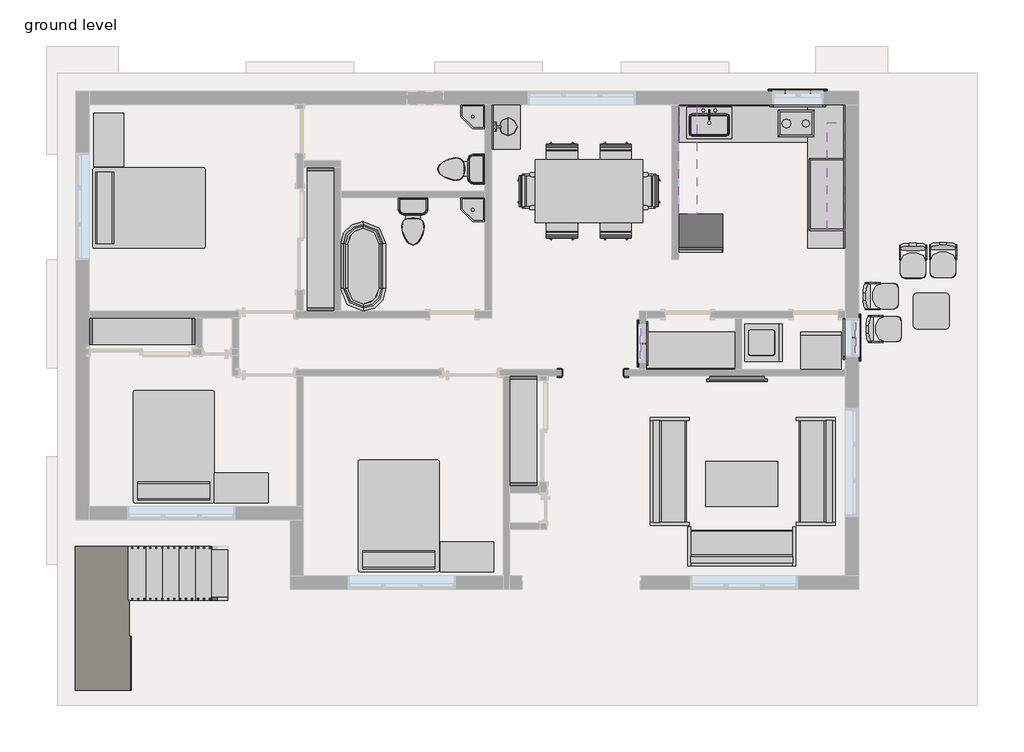
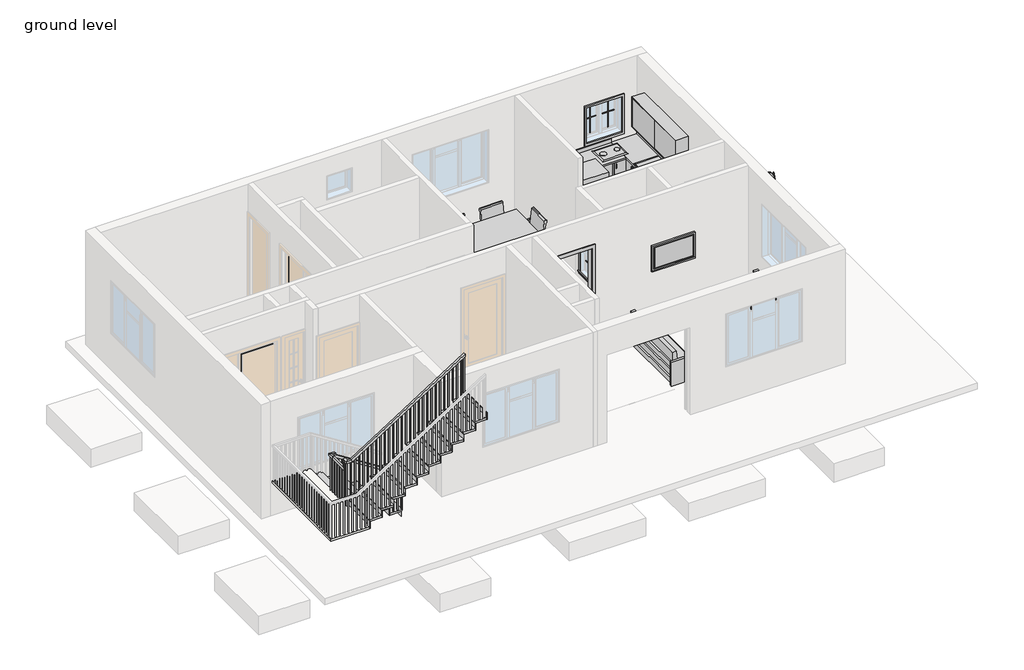
# One storey, part 4 of 4: 34 furniture elements, 17 proxies, 7 flow terminals, 2 stair flights, 1 railing, 1 slab.
"""IFC4 building model written with IfcOpenShell, lengths in millimetres."""

from ifc_helpers import new_model, si_unit, frame, origin, place, context, project, spatial, polyline, outline, extrude, faceted_brep, transform, mapped, element, save
from components import proxy_3c1fa1d0, proxy_97c73763, muntin_pattern_2x2_muntin_pattern_2x2_b3fe6957, muntin_pattern_2x2_muntin_pattern_2x2_3e0ecaf2, muntin_pattern_2x2_muntin_pattern_2x2_c35c595f, muntin_pattern_2x2_muntin_pattern_2x2_183aef24, proxy_bc9927fa, proxy_e6cf46b9, trim_window_exterior_flat_with_sill_41619996, trim_window_exterior_flat_with_sill_e38017c9, trim_window_exterior_flat_with_sill_5e960bf5, trim_window_interior_flat_picture_frame_51c85655, trim_window_interior_flat_picture_frame_d728ed12, trim_window_interior_flat_picture_frame_80babb00, proxy_1934c8a4, flow_terminal_15267b2a, flow_terminal_5b58e753, flow_terminal_4d548711, toilet_domestic_3d_toilet_domestic_3d_ba6479b0, toilet_domestic_3d_toilet_domestic_3d_30431060, flow_terminal_ce36f001, furniture_48488436, furniture_f87f75a4, furniture_97fe820d, furniture_52ef1662, furniture_6b884072, chair_task_chair_task_b7f3823b, chair_task_arms_chair_task_arms_fa5a08ef, furniture_deb1c5d1, furniture_9388d8e7, furniture_74614b7d, furniture_eb3a3c23, furniture_53a00f75, furniture_df918c0e, furniture_57be741f, furniture_57f9710a, furniture_acc2807d, furniture_65ba067b, furniture_5d68651d, furniture_b6aab1a0, furniture_1cc80a06, non_monolithic_landing_1ab817cb, stair_flight_17170d3d, stair_flight_b41fd25d

model = new_model("IFC4")

# Units and contexts
model_context = context("Model", 3, world=origin())
ifc_project = project(units=[si_unit("LENGTHUNIT", "METRE", prefix="MILLI")], contexts=[model_context])

# Site, building, storey
site = spatial("IfcSite", under=ifc_project)
building = spatial("IfcBuilding", under=site)
storey = spatial("IfcBuildingStorey", under=building, Name="ground level", Elevation=609.6)

# Proxies
placement = place(None, origin())
proxy_shape = proxy_3c1fa1d0(model_context)
element("IfcBuildingElementProxy", 1, Name="Cook Top-2 Unit : 12\" x 18\"", ObjectType="Cook Top-2 Unit : 12\" x 18\"", at=placement, inside=storey, context=model_context, shape_type="MappedRepresentation", body=[
    mapped(proxy_shape, transform((3099.7984427, 6060.3661978, 609.6), x_axis=(0.0, 1.0, 0.0), y_axis=(-1.0, 0.0, 0.0), z_axis=(0.0, 0.0, 1.0))),
])
proxy_2_shape = proxy_97c73763(model_context)
element("IfcBuildingElementProxy", 2, Name="Dryer : 27\" x 25\" x 35\"", ObjectType="Dryer : 27\" x 25\" x 35\"", at=placement, inside=storey, context=model_context, shape_type="MappedRepresentation", body=[
    mapped(proxy_2_shape, transform((3116.0361908, 1961.105194, 609.6), x_axis=(1.0, 0.0, 0.0), y_axis=(0.0, 1.0, 0.0), z_axis=(0.0, 0.0, 1.0))),
])
muntin_pattern_2x2_muntin_pattern_2x2_shape = muntin_pattern_2x2_muntin_pattern_2x2_b3fe6957(model_context)
element("IfcBuildingElementProxy", 3, Name="Muntin Pattern_2x2 : Muntin Pattern_2x2", ObjectType="Muntin Pattern_2x2 : Muntin Pattern_2x2", at=placement, inside=storey, context=model_context, shape_type="MappedRepresentation", body=[
    mapped(muntin_pattern_2x2_muntin_pattern_2x2_shape, transform((2887.0111471, 6673.1411978, 1771.65), x_axis=(1.0, 0.0, 0.0), y_axis=(0.0, 1.0, 0.0), z_axis=(0.0, 0.0, 1.0))),
])
muntin_pattern_2x2_muntin_pattern_2x2_2_shape = muntin_pattern_2x2_muntin_pattern_2x2_3e0ecaf2(model_context)
element("IfcBuildingElementProxy", 4, Name="Muntin Pattern_2x2 : Muntin Pattern_2x2", ObjectType="Muntin Pattern_2x2 : Muntin Pattern_2x2", at=placement, inside=storey, context=model_context, shape_type="MappedRepresentation", body=[
    mapped(muntin_pattern_2x2_muntin_pattern_2x2_2_shape, transform((3315.6361471, 6673.1411978, 1771.65), x_axis=(-1.0, 0.0, 0.0), y_axis=(0.0, -1.0, 0.0), z_axis=(0.0, 0.0, 1.0))),
])
muntin_pattern_2x2_muntin_pattern_2x2_3_shape = muntin_pattern_2x2_muntin_pattern_2x2_c35c595f(model_context)
element("IfcBuildingElementProxy", 5, Name="Muntin Pattern_2x2 : Muntin Pattern_2x2", ObjectType="Muntin Pattern_2x2 : Muntin Pattern_2x2", at=placement, inside=storey, context=model_context, shape_type="MappedRepresentation", body=[
    mapped(muntin_pattern_2x2_muntin_pattern_2x2_3_shape, transform((4095.0986471, 2498.0161978, 2079.625), x_axis=(0.0, -1.0, 0.0), y_axis=(1.0, 0.0, 0.0), z_axis=(0.0, 0.0, 1.0))),
])
element("IfcBuildingElementProxy", 6, Name="Muntin Pattern_2x2 : Muntin Pattern_2x2", ObjectType="Muntin Pattern_2x2 : Muntin Pattern_2x2", at=placement, inside=storey, context=model_context, shape_type="MappedRepresentation", body=[
    mapped(muntin_pattern_2x2_muntin_pattern_2x2_3_shape, transform((4050.6486471, 2498.0161978, 1600.2), x_axis=(0.0, -1.0, 0.0), y_axis=(1.0, 0.0, 0.0), z_axis=(0.0, 0.0, 1.0))),
])
muntin_pattern_2x2_muntin_pattern_2x2_4_shape = muntin_pattern_2x2_muntin_pattern_2x2_183aef24(model_context)
element("IfcBuildingElementProxy", 7, Name="Muntin Pattern_2x2 : Muntin Pattern_2x2", ObjectType="Muntin Pattern_2x2 : Muntin Pattern_2x2", at=placement, inside=storey, context=model_context, shape_type="MappedRepresentation", body=[
    mapped(muntin_pattern_2x2_muntin_pattern_2x2_4_shape, transform((443.8486471, 2396.4161978, 2079.625), x_axis=(0.0, -1.0, 0.0), y_axis=(1.0, 0.0, 0.0), z_axis=(0.0, 0.0, 1.0))),
])
element("IfcBuildingElementProxy", 8, Name="Muntin Pattern_2x2 : Muntin Pattern_2x2", ObjectType="Muntin Pattern_2x2 : Muntin Pattern_2x2", at=placement, inside=storey, context=model_context, shape_type="MappedRepresentation", body=[
    mapped(muntin_pattern_2x2_muntin_pattern_2x2_4_shape, transform((488.2986471, 2396.4161978, 1600.2), x_axis=(0.0, -1.0, 0.0), y_axis=(1.0, 0.0, 0.0), z_axis=(0.0, 0.0, 1.0))),
])
proxy_3_shape = proxy_bc9927fa(model_context)
element("IfcBuildingElementProxy", 9, Name="Passage Opening-Cased : 36\" x 84\"", ObjectType="Passage Opening-Cased : 36\" x 84\"", at=placement, inside=storey, context=model_context, shape_type="MappedRepresentation", body=[
    mapped(proxy_3_shape, transform((-386.6650096, 1901.1161978, 609.6), x_axis=(-1.0, 0.0, 0.0), y_axis=(0.0, -1.0, 0.0), z_axis=(0.0, 0.0, 1.0))),
])
proxy_4_shape = proxy_e6cf46b9(model_context)
element("IfcBuildingElementProxy", 10, Name="Refrigerator-Built-in : 30\" x 24\" RH", ObjectType="Refrigerator-Built-in : 30\" x 24\" RH", at=placement, inside=storey, context=model_context, shape_type="MappedRepresentation", body=[
    mapped(proxy_4_shape, transform((1450.3236471, 4309.7422263, 609.6), x_axis=(1.0, 0.0, 0.0), y_axis=(0.0, 1.0, 0.0), z_axis=(0.0, 0.0, 1.0))),
])
trim_window_exterior_flat_with_sill_shape = trim_window_exterior_flat_with_sill_41619996(model_context)
element("IfcBuildingElementProxy", 11, Name="Trim-Window-Exterior-Flat : with Sill", ObjectType="Trim-Window-Exterior-Flat : with Sill", at=placement, inside=storey, context=model_context, shape_type="MappedRepresentation", body=[
    mapped(trim_window_exterior_flat_with_sill_shape, transform((3101.3236471, 6682.6661978, 2616.2), x_axis=(-1.0, 0.0, 0.0), y_axis=(0.0, 0.0, 1.0), z_axis=(0.0, 1.0, 0.0))),
])
trim_window_exterior_flat_with_sill_2_shape = trim_window_exterior_flat_with_sill_e38017c9(model_context)
element("IfcBuildingElementProxy", 12, Name="Trim-Window-Exterior-Flat : with Sill", ObjectType="Trim-Window-Exterior-Flat : with Sill", at=placement, inside=storey, context=model_context, shape_type="MappedRepresentation", body=[
    mapped(trim_window_exterior_flat_with_sill_2_shape, transform((4130.0236471, 2498.0161978, 2590.8), x_axis=(0.0, 1.0, 0.0), y_axis=(0.0, 0.0, 1.0), z_axis=(1.0, 0.0, 0.0))),
])
trim_window_exterior_flat_with_sill_3_shape = trim_window_exterior_flat_with_sill_5e960bf5(model_context)
element("IfcBuildingElementProxy", 13, Name="Trim-Window-Exterior-Flat : with Sill", ObjectType="Trim-Window-Exterior-Flat : with Sill", at=placement, inside=storey, context=model_context, shape_type="MappedRepresentation", body=[
    mapped(trim_window_exterior_flat_with_sill_3_shape, transform((408.9236471, 2396.4161978, 2590.8), x_axis=(0.0, 1.0, 0.0), y_axis=(0.0, 0.0, -1.0), z_axis=(-1.0, 0.0, 0.0))),
])
trim_window_interior_flat_picture_frame_shape = trim_window_interior_flat_picture_frame_51c85655(model_context)
element("IfcBuildingElementProxy", 14, Name="Trim-Window-Interior-Flat : Picture Frame", ObjectType="Trim-Window-Interior-Flat : Picture Frame", at=placement, inside=storey, context=model_context, shape_type="MappedRepresentation", body=[
    mapped(trim_window_interior_flat_picture_frame_shape, transform((3101.3236471, 6454.0661978, 2616.2), x_axis=(1.0, 0.0, 0.0), y_axis=(0.0, 0.0, 1.0), z_axis=(0.0, -1.0, 0.0))),
])
trim_window_interior_flat_picture_frame_2_shape = trim_window_interior_flat_picture_frame_d728ed12(model_context)
element("IfcBuildingElementProxy", 15, Name="Trim-Window-Interior-Flat : Picture Frame", ObjectType="Trim-Window-Interior-Flat : Picture Frame", at=placement, inside=storey, context=model_context, shape_type="MappedRepresentation", body=[
    mapped(trim_window_interior_flat_picture_frame_2_shape, transform((3901.4236471, 2498.0161978, 2590.8), x_axis=(0.0, -1.0, 0.0), y_axis=(0.0, 0.0, 1.0), z_axis=(-1.0, 0.0, 0.0))),
])
trim_window_interior_flat_picture_frame_3_shape = trim_window_interior_flat_picture_frame_80babb00(model_context)
element("IfcBuildingElementProxy", 16, Name="Trim-Window-Interior-Flat : Picture Frame", ObjectType="Trim-Window-Interior-Flat : Picture Frame", at=placement, inside=storey, context=model_context, shape_type="MappedRepresentation", body=[
    mapped(trim_window_interior_flat_picture_frame_3_shape, transform((523.2236471, 2396.4161978, 2590.8), x_axis=(0.0, -1.0, 0.0), y_axis=(0.0, 0.0, -1.0), z_axis=(1.0, 0.0, 0.0))),
])
proxy_5_shape = proxy_1934c8a4(model_context)
element("IfcBuildingElementProxy", 17, Name="Washer : 25\" x 25\" x 35\"", ObjectType="Washer : 25\" x 25\" x 35\"", at=placement, inside=storey, context=model_context, shape_type="MappedRepresentation", body=[
    mapped(proxy_5_shape, transform((2237.9740823, 2809.1661978, 609.6), x_axis=(0.0, -1.0, 0.0), y_axis=(1.0, 0.0, 0.0), z_axis=(0.0, 0.0, 1.0))),
])

# Flow terminals
flow_terminal_shape = flow_terminal_15267b2a(model_context)
element("IfcFlowTerminal", 18, ObjectType="Lavatory - Vanity : 30\"x18\" - Private", at=placement, inside=storey, context=model_context, shape_type="MappedRepresentation", body=[
    mapped(flow_terminal_shape, transform((-2099.3263529, 6079.4161978, 609.6), x_axis=(1.0, 0.0, 0.0), y_axis=(0.0, 1.0, 0.0), z_axis=(0.0, 0.0, 1.0))),
])
flow_terminal_2_shape = flow_terminal_5b58e753(model_context)
element("IfcFlowTerminal", 19, ObjectType="Sink - Mop : 28\"x28\"", at=placement, inside=storey, context=model_context, shape_type="MappedRepresentation", body=[
    mapped(flow_terminal_2_shape, transform((-2213.6263529, 4872.9161978, 609.6), x_axis=(0.0, -1.0, 0.0), y_axis=(1.0, 0.0, 0.0), z_axis=(0.0, 0.0, 1.0))),
])
element("IfcFlowTerminal", 20, ObjectType="Sink - Mop : 28\"x28\"", at=placement, inside=storey, context=model_context, shape_type="MappedRepresentation", body=[
    mapped(flow_terminal_2_shape, transform((-2213.6263529, 6454.0661978, 609.6), x_axis=(0.0, -1.0, 0.0), y_axis=(1.0, 0.0, 0.0), z_axis=(0.0, 0.0, 1.0))),
])
flow_terminal_3_shape = flow_terminal_4d548711(model_context)
element("IfcFlowTerminal", 21, ObjectType="Sink Kitchen-Single : 30\" x 21\"", at=placement, inside=storey, context=model_context, shape_type="MappedRepresentation", body=[
    mapped(flow_terminal_3_shape, transform((1580.6844065, 6146.9207967, 609.6), x_axis=(1.0, 0.0, 0.0), y_axis=(0.0, 1.0, 0.0), z_axis=(0.0, 0.0, 1.0))),
])
toilet_domestic_3d_toilet_domestic_3d_shape = toilet_domestic_3d_toilet_domestic_3d_ba6479b0(model_context)
toilet_domestic_3d_toilet_domestic_3d_2_shape = toilet_domestic_3d_toilet_domestic_3d_30431060(model_context)
element("IfcFlowTerminal", 22, ObjectType="Toilet-Domestic-3D : Toilet-Domestic-3D", at=placement, inside=storey, context=model_context, shape_type="MappedRepresentation", body=[
    mapped(toilet_domestic_3d_toilet_domestic_3d_shape, transform((-3433.7493286, 4378.2201704, 609.6), x_axis=(1.0, 0.0, 0.0), y_axis=(0.0, 1.0, 0.0), z_axis=(0.0, 0.0, 1.0))),
    mapped(toilet_domestic_3d_toilet_domestic_3d_2_shape, transform((-3433.7493286, 4378.2201704, 609.6), x_axis=(1.0, 0.0, 0.0), y_axis=(0.0, 1.0, 0.0), z_axis=(0.0, 0.0, 1.0))),
])
element("IfcFlowTerminal", 23, ObjectType="Toilet-Domestic-3D : Toilet-Domestic-3D", at=placement, inside=storey, context=model_context, shape_type="MappedRepresentation", body=[
    mapped(toilet_domestic_3d_toilet_domestic_3d_shape, transform((-2708.3223803, 5361.8661978, 609.6), x_axis=(0.0, -1.0, 0.0), y_axis=(1.0, 0.0, 0.0), z_axis=(0.0, 0.0, 1.0))),
    mapped(toilet_domestic_3d_toilet_domestic_3d_2_shape, transform((-2708.3223803, 5361.8661978, 609.6), x_axis=(0.0, -1.0, 0.0), y_axis=(1.0, 0.0, 0.0), z_axis=(0.0, 0.0, 1.0))),
])
flow_terminal_4_shape = flow_terminal_ce36f001(model_context)
element("IfcFlowTerminal", 24, ObjectType="Tub-Free Standing-3D : 30\" x 60\"", at=placement, inside=storey, context=model_context, shape_type="MappedRepresentation", body=[
    mapped(flow_terminal_4_shape, transform((-4277.3763529, 3710.8661978, 609.6), x_axis=(-1.0, 0.0, 0.0), y_axis=(0.0, -1.0, 0.0), z_axis=(0.0, 0.0, 1.0))),
])

# Furniture
furniture_shape = furniture_48488436(model_context)
element("IfcFurniture", 25, ObjectType="48\"", at=placement, inside=storey, context=model_context, shape_type="MappedRepresentation", body=[
    mapped(furniture_shape, transform((3901.4236471, 5020.9111578, 609.6), x_axis=(0.0, -1.0, 0.0), y_axis=(1.0, 0.0, 0.0), z_axis=(0.0, 0.0, 1.0))),
])
furniture_2_shape = furniture_f87f75a4(model_context)
element("IfcFurniture", 26, ObjectType="Base Cabinet-Combo01 : 30\"", at=placement, inside=storey, context=model_context, shape_type="MappedRepresentation", body=[
    mapped(furniture_2_shape, transform((2587.2859422, 6454.0661978, 609.6), x_axis=(1.0, 0.0, 0.0), y_axis=(0.0, 1.0, 0.0), z_axis=(0.0, 0.0, 1.0))),
])
furniture_3_shape = furniture_97fe820d(model_context)
element("IfcFurniture", 27, ObjectType="Base Cabinet-Corner Unit-Square : 36\"", at=placement, inside=storey, context=model_context, shape_type="MappedRepresentation", body=[
    mapped(furniture_3_shape, transform((3374.6859422, 6454.0661978, 609.6), x_axis=(1.0, 0.0, 0.0), y_axis=(0.0, 1.0, 0.0), z_axis=(0.0, 0.0, 1.0))),
])
furniture_4_shape = furniture_52ef1662(model_context)
element("IfcFurniture", 28, ObjectType="Bed-Standard : Double 54\" x 75\"", at=placement, inside=storey, context=model_context, shape_type="MappedRepresentation", body=[
    mapped(furniture_4_shape, transform((-7961.5214349, 4429.9776732, 609.6), x_axis=(0.0, 1.0, 0.0), y_axis=(-1.0, 0.0, 0.0), z_axis=(0.0, 0.0, 1.0))),
])
element("IfcFurniture", 29, ObjectType="Bed-Standard : Double 54\" x 75\"", at=placement, inside=storey, context=model_context, shape_type="MappedRepresentation", body=[
    mapped(furniture_4_shape, transform((-7225.3378283, 598.2211158, 609.6), x_axis=(-1.0, 0.0, 0.0), y_axis=(0.0, -1.0, 0.0), z_axis=(0.0, 0.0, 1.0))),
])
element("IfcFurniture", 30, ObjectType="Bed-Standard : Double 54\" x 75\"", at=placement, inside=storey, context=model_context, shape_type="MappedRepresentation", body=[
    mapped(furniture_4_shape, transform((-3402.6378283, -576.5288842, 609.6), x_axis=(-1.0, 0.0, 0.0), y_axis=(0.0, -1.0, 0.0), z_axis=(0.0, 0.0, 1.0))),
])
furniture_5_shape = furniture_6b884072(model_context)
element("IfcFurniture", 31, ObjectType="Cabinet File-Lateral 2 Drawer : 36\" x 20\" x 24\"", at=placement, inside=storey, context=model_context, shape_type="MappedRepresentation", body=[
    mapped(furniture_5_shape, transform((-9536.044729, 6037.1887117, 609.6), x_axis=(0.0, 1.0, 0.0), y_axis=(-1.0, 0.0, 0.0), z_axis=(0.0, 0.0, 1.0))),
])
element("IfcFurniture", 32, ObjectType="Cabinet File-Lateral 2 Drawer : 36\" x 20\" x 24\"", at=placement, inside=storey, context=model_context, shape_type="MappedRepresentation", body=[
    mapped(furniture_5_shape, transform((-6527.4988668, -989.0021783, 609.6), x_axis=(-1.0, 0.0, 0.0), y_axis=(0.0, -1.0, 0.0), z_axis=(0.0, 0.0, 1.0))),
])
element("IfcFurniture", 33, ObjectType="Cabinet File-Lateral 2 Drawer : 36\" x 20\" x 24\"", at=placement, inside=storey, context=model_context, shape_type="MappedRepresentation", body=[
    mapped(furniture_5_shape, transform((-2698.4488668, -2163.7521783, 609.6), x_axis=(-1.0, 0.0, 0.0), y_axis=(0.0, -1.0, 0.0), z_axis=(0.0, 0.0, 1.0))),
])
chair_task_chair_task_shape = chair_task_chair_task_b7f3823b(model_context)
element("IfcFurniture", 34, ObjectType="Chair-Task : Chair-Task", at=placement, inside=storey, context=model_context, shape_type="MappedRepresentation", body=[
    mapped(chair_task_chair_task_shape, transform((149.8644668, 5539.5620994, 609.6), x_axis=(-1.0, 0.0, 0.0), y_axis=(0.0, -1.0, 0.0), z_axis=(0.0, 0.0, 1.0))),
])
element("IfcFurniture", 35, ObjectType="Chair-Task : Chair-Task", at=placement, inside=storey, context=model_context, shape_type="MappedRepresentation", body=[
    mapped(chair_task_chair_task_shape, transform((-132.1171726, 4434.8702962, 609.6), x_axis=(1.0, 0.0, 0.0), y_axis=(0.0, 1.0, 0.0), z_axis=(0.0, 0.0, 1.0))),
])
element("IfcFurniture", 36, ObjectType="Chair-Task : Chair-Task", at=placement, inside=storey, context=model_context, shape_type="MappedRepresentation", body=[
    mapped(chair_task_chair_task_shape, transform((-764.5355332, 5539.5620994, 609.6), x_axis=(-1.0, 0.0, 0.0), y_axis=(0.0, -1.0, 0.0), z_axis=(0.0, 0.0, 1.0))),
])
element("IfcFurniture", 37, ObjectType="Chair-Task : Chair-Task", at=placement, inside=storey, context=model_context, shape_type="MappedRepresentation", body=[
    mapped(chair_task_chair_task_shape, transform((-1046.5171726, 4434.8702962, 609.6), x_axis=(1.0, 0.0, 0.0), y_axis=(0.0, 1.0, 0.0), z_axis=(0.0, 0.0, 1.0))),
])
chair_task_arms_chair_task_arms_shape = chair_task_arms_chair_task_arms_fa5a08ef(model_context)
element("IfcFurniture", 38, ObjectType="Chair-Task Arms : Chair-Task Arms", at=placement, inside=storey, context=model_context, shape_type="MappedRepresentation", body=[
    mapped(chair_task_arms_chair_task_arms_shape, transform((-1381.6722545, 5128.2070175, 609.6), x_axis=(0.0, -1.0, 0.0), y_axis=(1.0, 0.0, 0.0), z_axis=(0.0, 0.0, 1.0))),
])
element("IfcFurniture", 39, ObjectType="Chair-Task Arms : Chair-Task Arms", at=placement, inside=storey, context=model_context, shape_type="MappedRepresentation", body=[
    mapped(chair_task_arms_chair_task_arms_shape, transform((485.0195487, 4846.2253781, 609.6), x_axis=(0.0, 1.0, 0.0), y_axis=(-1.0, 0.0, 0.0), z_axis=(0.0, 0.0, 1.0))),
])
furniture_6_shape = furniture_deb1c5d1(model_context)
element("IfcFurniture", 40, ObjectType="Counter Top : 24\" Depth", at=placement, inside=storey, context=model_context, shape_type="MappedRepresentation", body=[
    mapped(furniture_6_shape, transform((3901.4236471, 5253.6039027, 609.6), x_axis=(0.0, -1.0, 0.0), y_axis=(1.0, 0.0, 0.0), z_axis=(0.0, 0.0, 1.0))),
])
furniture_7_shape = furniture_9388d8e7(model_context)
element("IfcFurniture", 41, ObjectType="Counter Top : 24\" Depth", at=placement, inside=storey, context=model_context, shape_type="MappedRepresentation", body=[
    mapped(furniture_7_shape, transform((834.061352, 1958.2661978, 609.6), x_axis=(-1.0, 0.0, 0.0), y_axis=(0.0, -1.0, 0.0), z_axis=(0.0, 0.0, 1.0))),
])
furniture_8_shape = furniture_74614b7d(model_context)
element("IfcFurniture", 42, ObjectType="Counter Top w Sink Hole : 24\" Depth", at=placement, inside=storey, context=model_context, shape_type="MappedRepresentation", body=[
    mapped(furniture_8_shape, transform((2276.1359422, 6454.0661978, 609.6), x_axis=(1.0, 0.0, 0.0), y_axis=(0.0, 1.0, 0.0), z_axis=(0.0, 0.0, 1.0))),
])
furniture_9_shape = furniture_eb3a3c23(model_context)
element("IfcFurniture", 43, ObjectType="Seating-Auditorium : 18\" x 24\" x 30\"", at=placement, inside=storey, context=model_context, shape_type="MappedRepresentation", body=[
    mapped(furniture_9_shape, transform((4308.4482373, 3363.5940666, 609.6), x_axis=(0.0, -1.0, 0.0), y_axis=(1.0, 0.0, 0.0), z_axis=(0.0, 0.0, 1.0))),
])
element("IfcFurniture", 44, ObjectType="Seating-Auditorium : 18\" x 24\" x 30\"", at=placement, inside=storey, context=model_context, shape_type="MappedRepresentation", body=[
    mapped(furniture_9_shape, transform((4359.2482373, 2804.7940666, 609.6), x_axis=(0.0, -1.0, 0.0), y_axis=(1.0, 0.0, 0.0), z_axis=(0.0, 0.0, 1.0))),
])
element("IfcFurniture", 45, ObjectType="Seating-Auditorium : 18\" x 24\" x 30\"", at=placement, inside=storey, context=model_context, shape_type="MappedRepresentation", body=[
    mapped(furniture_9_shape, transform((5217.8515159, 4002.3416076, 609.6), x_axis=(-1.0, 0.0, 0.0), y_axis=(0.0, -1.0, 0.0), z_axis=(0.0, 0.0, 1.0))),
])
element("IfcFurniture", 46, ObjectType="Seating-Auditorium : 18\" x 24\" x 30\"", at=placement, inside=storey, context=model_context, shape_type="MappedRepresentation", body=[
    mapped(furniture_9_shape, transform((5725.8515159, 4015.0416076, 609.6), x_axis=(-1.0, 0.0, 0.0), y_axis=(0.0, -1.0, 0.0), z_axis=(0.0, 0.0, 1.0))),
])
furniture_10_shape = furniture_53a00f75(model_context)
element("IfcFurniture", 47, ObjectType="Shelving : 96\" x 12\" x 84\"", at=placement, inside=storey, context=model_context, shape_type="MappedRepresentation", body=[
    mapped(furniture_10_shape, transform((-1864.3763529, 910.5161978, 609.6), x_axis=(0.0, 1.0, 0.0), y_axis=(-1.0, 0.0, 0.0), z_axis=(0.0, 0.0, 1.0))),
])
furniture_11_shape = furniture_df918c0e(model_context)
element("IfcFurniture", 48, ObjectType="Shelving : 96\" x 12\" x 84\" 2", at=placement, inside=storey, context=model_context, shape_type="MappedRepresentation", body=[
    mapped(furniture_11_shape, transform((-8030.2263529, 2910.7661978, 609.6), x_axis=(1.0, 0.0, 0.0), y_axis=(0.0, 1.0, 0.0), z_axis=(0.0, 0.0, 1.0))),
])
furniture_12_shape = furniture_57be741f(model_context)
element("IfcFurniture", 49, ObjectType="Shelving : 96\" x 12\" x 84\" 3", at=placement, inside=storey, context=model_context, shape_type="MappedRepresentation", body=[
    mapped(furniture_12_shape, transform((-5306.0763529, 4168.0661978, 609.6), x_axis=(0.0, 1.0, 0.0), y_axis=(-1.0, 0.0, 0.0), z_axis=(0.0, 0.0, 1.0))),
])
furniture_13_shape = furniture_57f9710a(model_context)
element("IfcFurniture", 50, ObjectType="Sofa : 72\"", at=placement, inside=storey, context=model_context, shape_type="MappedRepresentation", body=[
    mapped(furniture_13_shape, transform((2219.1941389, -905.4797038, 609.6), x_axis=(-1.0, 0.0, 0.0), y_axis=(0.0, -1.0, 0.0), z_axis=(0.0, 0.0, 1.0))),
])
element("IfcFurniture", 51, ObjectType="Sofa : 72\"", at=placement, inside=storey, context=model_context, shape_type="MappedRepresentation", body=[
    mapped(furniture_13_shape, transform((3259.9695487, 295.0866896, 609.6), x_axis=(0.0, -1.0, 0.0), y_axis=(1.0, 0.0, 0.0), z_axis=(0.0, 0.0, 1.0))),
])
element("IfcFurniture", 52, ObjectType="Sofa : 72\"", at=placement, inside=storey, context=model_context, shape_type="MappedRepresentation", body=[
    mapped(furniture_13_shape, transform((1069.4277455, 154.345706, 609.6), x_axis=(0.0, 1.0, 0.0), y_axis=(-1.0, 0.0, 0.0), z_axis=(0.0, 0.0, 1.0))),
])
furniture_14_shape = furniture_acc2807d(model_context)
element("IfcFurniture", 53, ObjectType="Table-Coffee Rectangular : 48\" x 30\"", at=placement, inside=storey, context=model_context, shape_type="MappedRepresentation", body=[
    mapped(furniture_14_shape, transform((1535.4900168, -354.444634, 609.6), x_axis=(1.0, 0.0, 0.0), y_axis=(0.0, 1.0, 0.0), z_axis=(0.0, 0.0, 1.0))),
])
furniture_15_shape = furniture_65ba067b(model_context)
element("IfcFurniture", 54, ObjectType="Table-Conference2 w Chairs : 40\" x 90\"", at=placement, inside=storey, context=model_context, shape_type="MappedRepresentation", body=[
    mapped(furniture_15_shape, transform((-448.3263529, 4987.2161978, 609.6), x_axis=(1.0, 0.0, 0.0), y_axis=(0.0, 1.0, 0.0), z_axis=(0.0, 0.0, 1.0))),
])
furniture_16_shape = furniture_5d68651d(model_context)
element("IfcFurniture", 55, ObjectType="Table-End : 24\" x 24\"", at=placement, inside=storey, context=model_context, shape_type="MappedRepresentation", body=[
    mapped(furniture_16_shape, transform((5053.3900168, 2796.4661978, 609.6), x_axis=(1.0, 0.0, 0.0), y_axis=(0.0, 1.0, 0.0), z_axis=(0.0, 0.0, 1.0))),
])
furniture_17_shape = furniture_b6aab1a0(model_context)
element("IfcFurniture", 56, ObjectType="Television-Plasma : 42\"", at=placement, inside=storey, context=model_context, shape_type="MappedRepresentation", body=[
    mapped(furniture_17_shape, transform((2009.1236471, 1843.9661978, 1676.4), x_axis=(1.0, 0.0, 0.0), y_axis=(0.0, 1.0, 0.0), z_axis=(0.0, 0.0, 1.0))),
])
furniture_18_shape = furniture_1cc80a06(model_context)
element("IfcFurniture", 57, ObjectType="Upper Cabinet-Pass-Thru w Glass : 48\" x 30\" x 12\"", at=placement, inside=storey, context=model_context, shape_type="MappedRepresentation", body=[
    mapped(furniture_18_shape, transform((1075.6736471, 5495.5284929, 609.6), x_axis=(0.0, 1.0, 0.0), y_axis=(-1.0, 0.0, 0.0), z_axis=(0.0, 0.0, 1.0))),
])
element("IfcFurniture", 58, ObjectType="Upper Cabinet-Pass-Thru w Glass : 48\" x 30\" x 12\"", at=placement, inside=storey, context=model_context, shape_type="MappedRepresentation", body=[
    mapped(furniture_18_shape, transform((3596.6236471, 5216.1284929, 609.6), x_axis=(0.0, 1.0, 0.0), y_axis=(-1.0, 0.0, 0.0), z_axis=(0.0, 0.0, 1.0))),
])

# Railing
element("IfcRailing", 59, ObjectType="Handrail - Rectangular", at=placement, inside=storey, context=model_context, shape_type="SolidModel", body=[
    faceted_brep([(-6576.0763529, -1966.0338022, 1701.8), (-6576.0763529, -1966.0338022, 1641.586276), (-6576.0763529, -1915.2338022, 1641.586276), (-6576.0763529, -1915.2338022, 1701.8), (-8176.2763529, -1966.0338022, 2720.1090909), (-8227.0763529, -1966.0338022, 2692.2226396), (-8227.0763529, -1915.2338022, 2692.2226396), (-8176.2763529, -1915.2338022, 2720.1090909), (-8176.2763529, -1966.0338022, 2768.6), (-8227.0763529, -1966.0338022, 2717.8), (-8227.0763529, -1915.2338022, 2717.8), (-8176.2763529, -1915.2338022, 2768.6), (-8252.4763529, -1966.0338022, 2768.6), (-8252.4763529, -1966.0338022, 2717.8), (-8303.2763529, -1915.2338022, 2717.8), (-8303.2763529, -1915.2338022, 2768.6), (-8252.4763529, -2042.2338022, 2768.6), (-8252.4763529, -2042.2338022, 2717.8), (-8303.2763529, -2042.2338022, 2717.8), (-8303.2763529, -2042.2338022, 2768.6), (-8252.4763529, -2499.4338022, 2768.6), (-8252.4763529, -2550.2338022, 2717.8), (-8303.2763529, -2550.2338022, 2717.8), (-8303.2763529, -2499.4338022, 2768.6), (-8252.4763529, -2499.4338022, 2994.8909091), (-8252.4763529, -2550.2338022, 2944.0909091), (-8303.2763529, -2550.2338022, 2944.0909091), (-8303.2763529, -2499.4338022, 2994.8909091), (-8252.4763529, -2575.6338022, 2994.8909091), (-8252.4763529, -2575.6338022, 2944.0909091), (-8303.2763529, -2626.4338022, 2944.0909091), (-8303.2763529, -2626.4338022, 2994.8909091), (-8176.2763529, -2575.6338022, 2994.8909091), (-8161.483358, -2575.6338022, 2944.0909091), (-8161.483358, -2626.4338022, 2944.0909091), (-8176.2763529, -2626.4338022, 2994.8909091), (-5458.4763529, -2575.6338022, 4724.4), (-5458.4763529, -2626.4338022, 4724.4), (-5458.4763529, -2626.4338022, 4664.186276), (-5458.4763529, -2575.6338022, 4664.186276)], [[[0, 1, 2, 3]], [[1, 0, 4, 5]], [[2, 1, 5, 6]], [[3, 2, 6, 7]], [[0, 3, 7, 4]], [[5, 4, 8, 9]], [[6, 5, 9, 10]], [[7, 6, 10, 11]], [[4, 7, 11, 8]], [[9, 8, 12, 13]], [[10, 9, 13, 14]], [[11, 10, 14, 15]], [[8, 11, 15, 12]], [[13, 12, 16, 17]], [[14, 13, 17, 18]], [[15, 14, 18, 19]], [[12, 15, 19, 16]], [[17, 16, 20, 21]], [[18, 17, 21, 22]], [[19, 18, 22, 23]], [[16, 19, 23, 20]], [[21, 20, 24, 25]], [[22, 21, 25, 26]], [[23, 22, 26, 27]], [[20, 23, 27, 24]], [[25, 24, 28, 29]], [[26, 25, 29, 30]], [[27, 26, 30, 31]], [[24, 27, 31, 28]], [[29, 28, 32, 33]], [[30, 29, 33, 34]], [[31, 30, 34, 35]], [[28, 31, 35, 32]], [[36, 37, 38, 39]], [[33, 32, 36, 39]], [[34, 33, 39, 38]], [[35, 34, 38, 37]], [[32, 35, 37, 36]]]),
    extrude(outline(polyline([(4609.6340032, -5544.2013529), (3632.2, -5544.2013529), (3632.2, -5525.1513529), (4621.7567305, -5525.1513529), (4609.6340032, -5544.2013529)])), frame((0.0, -2610.5588022, 0.0), z_axis=(0.0, 1.0, 0.0), x_axis=(0.0, 0.0, 1.0)), (0.0, 0.0, 1.0), 19.05),
    extrude(outline(polyline([(4544.9794578, -5645.8013529), (3632.2, -5645.8013529), (3632.2, -5626.7513529), (4557.1021851, -5626.7513529), (4544.9794578, -5645.8013529)])), frame((0.0, -2610.5588022, 0.0), z_axis=(0.0, 1.0, 0.0), x_axis=(0.0, 0.0, 1.0)), (0.0, 0.0, 1.0), 19.05),
    extrude(outline(polyline([(4480.3249123, -5747.4013529), (3632.2, -5747.4013529), (3632.2, -5728.3513529), (4492.4476396, -5728.3513529), (4480.3249123, -5747.4013529)])), frame((0.0, -2610.5588022, 0.0), z_axis=(0.0, 1.0, 0.0), x_axis=(0.0, 0.0, 1.0)), (0.0, 0.0, 1.0), 19.05),
    extrude(outline(polyline([(4415.6703669, -5849.0013529), (3454.4, -5849.0013529), (3454.4, -5829.9513529), (4427.7930941, -5829.9513529), (4415.6703669, -5849.0013529)])), frame((0.0, -2610.5588022, 0.0), z_axis=(0.0, 1.0, 0.0), x_axis=(0.0, 0.0, 1.0)), (0.0, 0.0, 1.0), 19.05),
    extrude(outline(polyline([(4351.0158214, -5950.6013529), (3454.4, -5950.6013529), (3454.4, -5931.5513529), (4363.1385487, -5931.5513529), (4351.0158214, -5950.6013529)])), frame((0.0, -2610.5588022, 0.0), z_axis=(0.0, 1.0, 0.0), x_axis=(0.0, 0.0, 1.0)), (0.0, 0.0, 1.0), 19.05),
    extrude(outline(polyline([(4286.361276, -6052.2013529), (3276.6, -6052.2013529), (3276.6, -6033.1513529), (4298.4840032, -6033.1513529), (4286.361276, -6052.2013529)])), frame((0.0, -2610.5588022, 0.0), z_axis=(0.0, 1.0, 0.0), x_axis=(0.0, 0.0, 1.0)), (0.0, 0.0, 1.0), 19.05),
    extrude(outline(polyline([(4221.7067305, -6153.8013529), (3276.6, -6153.8013529), (3276.6, -6134.7513529), (4233.8294578, -6134.7513529), (4221.7067305, -6153.8013529)])), frame((0.0, -2610.5588022, 0.0), z_axis=(0.0, 1.0, 0.0), x_axis=(0.0, 0.0, 1.0)), (0.0, 0.0, 1.0), 19.05),
    extrude(outline(polyline([(4157.0521851, -6255.4013529), (3276.6, -6255.4013529), (3276.6, -6236.3513529), (4169.1749123, -6236.3513529), (4157.0521851, -6255.4013529)])), frame((0.0, -2610.5588022, 0.0), z_axis=(0.0, 1.0, 0.0), x_axis=(0.0, 0.0, 1.0)), (0.0, 0.0, 1.0), 19.05),
    extrude(outline(polyline([(4092.3976396, -6357.0013529), (3098.8, -6357.0013529), (3098.8, -6337.9513529), (4104.5203669, -6337.9513529), (4092.3976396, -6357.0013529)])), frame((0.0, -2610.5588022, 0.0), z_axis=(0.0, 1.0, 0.0), x_axis=(0.0, 0.0, 1.0)), (0.0, 0.0, 1.0), 19.05),
    extrude(outline(polyline([(4027.7430941, -6458.6013529), (3098.8, -6458.6013529), (3098.8, -6439.5513529), (4039.8658214, -6439.5513529), (4027.7430941, -6458.6013529)])), frame((0.0, -2610.5588022, 0.0), z_axis=(0.0, 1.0, 0.0), x_axis=(0.0, 0.0, 1.0)), (0.0, 0.0, 1.0), 19.05),
    extrude(outline(polyline([(3963.0885487, -6560.2013529), (3098.8, -6560.2013529), (3098.8, -6541.1513529), (3975.211276, -6541.1513529), (3963.0885487, -6560.2013529)])), frame((0.0, -2610.5588022, 0.0), z_axis=(0.0, 1.0, 0.0), x_axis=(0.0, 0.0, 1.0)), (0.0, 0.0, 1.0), 19.05),
    extrude(outline(polyline([(3898.4340032, -6661.8013529), (2921.0, -6661.8013529), (2921.0, -6642.7513529), (3910.5567305, -6642.7513529), (3898.4340032, -6661.8013529)])), frame((0.0, -2610.5588022, 0.0), z_axis=(0.0, 1.0, 0.0), x_axis=(0.0, 0.0, 1.0)), (0.0, 0.0, 1.0), 19.05),
    extrude(outline(polyline([(3833.7794578, -6763.4013529), (2921.0, -6763.4013529), (2921.0, -6744.3513529), (3845.9021851, -6744.3513529), (3833.7794578, -6763.4013529)])), frame((0.0, -2610.5588022, 0.0), z_axis=(0.0, 1.0, 0.0), x_axis=(0.0, 0.0, 1.0)), (0.0, 0.0, 1.0), 19.05),
    extrude(outline(polyline([(3769.1249123, -6865.0013529), (2921.0, -6865.0013529), (2921.0, -6845.9513529), (3781.2476396, -6845.9513529), (3769.1249123, -6865.0013529)])), frame((0.0, -2610.5588022, 0.0), z_axis=(0.0, 1.0, 0.0), x_axis=(0.0, 0.0, 1.0)), (0.0, 0.0, 1.0), 19.05),
    extrude(outline(polyline([(3704.4703669, -6966.6013529), (2743.2, -6966.6013529), (2743.2, -6947.5513529), (3716.5930941, -6947.5513529), (3704.4703669, -6966.6013529)])), frame((0.0, -2610.5588022, 0.0), z_axis=(0.0, 1.0, 0.0), x_axis=(0.0, 0.0, 1.0)), (0.0, 0.0, 1.0), 19.05),
    extrude(outline(polyline([(3639.8158214, -7068.2013529), (2743.2, -7068.2013529), (2743.2, -7049.1513529), (3651.9385487, -7049.1513529), (3639.8158214, -7068.2013529)])), frame((0.0, -2610.5588022, 0.0), z_axis=(0.0, 1.0, 0.0), x_axis=(0.0, 0.0, 1.0)), (0.0, 0.0, 1.0), 19.05),
    extrude(outline(polyline([(3575.161276, -7169.8013529), (2565.4, -7169.8013529), (2565.4, -7150.7513529), (3587.2840032, -7150.7513529), (3575.161276, -7169.8013529)])), frame((0.0, -2610.5588022, 0.0), z_axis=(0.0, 1.0, 0.0), x_axis=(0.0, 0.0, 1.0)), (0.0, 0.0, 1.0), 19.05),
    extrude(outline(polyline([(3510.5067305, -7271.4013529), (2565.4, -7271.4013529), (2565.4, -7252.3513529), (3522.6294578, -7252.3513529), (3510.5067305, -7271.4013529)])), frame((0.0, -2610.5588022, 0.0), z_axis=(0.0, 1.0, 0.0), x_axis=(0.0, 0.0, 1.0)), (0.0, 0.0, 1.0), 19.05),
    extrude(outline(polyline([(3445.8521851, -7373.0013529), (2565.4, -7373.0013529), (2565.4, -7353.9513529), (3457.9749123, -7353.9513529), (3445.8521851, -7373.0013529)])), frame((0.0, -2610.5588022, 0.0), z_axis=(0.0, 1.0, 0.0), x_axis=(0.0, 0.0, 1.0)), (0.0, 0.0, 1.0), 19.05),
    extrude(outline(polyline([(3381.1976396, -7474.6013529), (2387.6, -7474.6013529), (2387.6, -7455.5513529), (3393.3203669, -7455.5513529), (3381.1976396, -7474.6013529)])), frame((0.0, -2610.5588022, 0.0), z_axis=(0.0, 1.0, 0.0), x_axis=(0.0, 0.0, 1.0)), (0.0, 0.0, 1.0), 19.05),
    extrude(outline(polyline([(3316.5430941, -7576.2013529), (2387.6, -7576.2013529), (2387.6, -7557.1513529), (3328.6658214, -7557.1513529), (3316.5430941, -7576.2013529)])), frame((0.0, -2610.5588022, 0.0), z_axis=(0.0, 1.0, 0.0), x_axis=(0.0, 0.0, 1.0)), (0.0, 0.0, 1.0), 19.05),
    extrude(outline(polyline([(3251.8885487, -7677.8013529), (2387.6, -7677.8013529), (2387.6, -7658.7513529), (3264.011276, -7658.7513529), (3251.8885487, -7677.8013529)])), frame((0.0, -2610.5588022, 0.0), z_axis=(0.0, 1.0, 0.0), x_axis=(0.0, 0.0, 1.0)), (0.0, 0.0, 1.0), 19.05),
    extrude(outline(polyline([(3187.2340032, -7779.4013529), (2209.8, -7779.4013529), (2209.8, -7760.3513529), (3199.3567305, -7760.3513529), (3187.2340032, -7779.4013529)])), frame((0.0, -2610.5588022, 0.0), z_axis=(0.0, 1.0, 0.0), x_axis=(0.0, 0.0, 1.0)), (0.0, 0.0, 1.0), 19.05),
    extrude(outline(polyline([(3122.5794578, -7881.0013529), (2209.8, -7881.0013529), (2209.8, -7861.9513529), (3134.7021851, -7861.9513529), (3122.5794578, -7881.0013529)])), frame((0.0, -2610.5588022, 0.0), z_axis=(0.0, 1.0, 0.0), x_axis=(0.0, 0.0, 1.0)), (0.0, 0.0, 1.0), 19.05),
    extrude(outline(polyline([(3057.9249123, -7982.6013529), (2209.8, -7982.6013529), (2209.8, -7963.5513529), (3070.0476396, -7963.5513529), (3057.9249123, -7982.6013529)])), frame((0.0, -2610.5588022, 0.0), z_axis=(0.0, 1.0, 0.0), x_axis=(0.0, 0.0, 1.0)), (0.0, 0.0, 1.0), 19.05),
    extrude(outline(polyline([(2993.2703669, -8084.2013529), (2032.0, -8084.2013529), (2032.0, -8065.1513529), (3005.3930941, -8065.1513529), (2993.2703669, -8084.2013529)])), frame((0.0, -2610.5588022, 0.0), z_axis=(0.0, 1.0, 0.0), x_axis=(0.0, 0.0, 1.0)), (0.0, 0.0, 1.0), 19.05),
    extrude(outline(polyline([(2928.6158214, -8185.8013529), (2032.0, -8185.8013529), (2032.0, -8166.7513529), (2940.7385487, -8166.7513529), (2928.6158214, -8185.8013529)])), frame((0.0, -2610.5588022, 0.0), z_axis=(0.0, 1.0, 0.0), x_axis=(0.0, 0.0, 1.0)), (0.0, 0.0, 1.0), 19.05),
    extrude(outline(polyline([(-8268.3513529, -2540.7088022), (-8268.3513529, -2559.7588022), (-8287.4013529, -2559.7588022), (-8287.4013529, -2540.7088022), (-8268.3513529, -2540.7088022)])), frame((0.0, 0.0, 1854.2), z_axis=(0.0, 0.0, 1.0), x_axis=(1.0, 0.0, 0.0)), (0.0, 0.0, 1.0), 1089.8909091),
    extrude(outline(polyline([(-8268.3513529, -2439.1088022), (-8268.3513529, -2458.1588022), (-8287.4013529, -2458.1588022), (-8287.4013529, -2439.1088022), (-8268.3513529, -2439.1088022)])), frame((0.0, 0.0, 1854.2), z_axis=(0.0, 0.0, 1.0), x_axis=(1.0, 0.0, 0.0)), (0.0, 0.0, 1.0), 863.6),
    extrude(outline(polyline([(-8268.3513529, -2337.5088022), (-8268.3513529, -2356.5588022), (-8287.4013529, -2356.5588022), (-8287.4013529, -2337.5088022), (-8268.3513529, -2337.5088022)])), frame((0.0, 0.0, 1854.2), z_axis=(0.0, 0.0, 1.0), x_axis=(1.0, 0.0, 0.0)), (0.0, 0.0, 1.0), 863.6),
    extrude(outline(polyline([(-8268.3513529, -2235.9088022), (-8268.3513529, -2254.9588022), (-8287.4013529, -2254.9588022), (-8287.4013529, -2235.9088022), (-8268.3513529, -2235.9088022)])), frame((0.0, 0.0, 1854.2), z_axis=(0.0, 0.0, 1.0), x_axis=(1.0, 0.0, 0.0)), (0.0, 0.0, 1.0), 863.6),
    extrude(outline(polyline([(-8268.3513529, -2134.3088022), (-8268.3513529, -2153.3588022), (-8287.4013529, -2153.3588022), (-8287.4013529, -2134.3088022), (-8268.3513529, -2134.3088022)])), frame((0.0, 0.0, 1854.2), z_axis=(0.0, 0.0, 1.0), x_axis=(1.0, 0.0, 0.0)), (0.0, 0.0, 1.0), 863.6),
    extrude(outline(polyline([(-8268.3513529, -2032.7088022), (-8268.3513529, -2051.7588022), (-8287.4013529, -2051.7588022), (-8287.4013529, -2032.7088022), (-8268.3513529, -2032.7088022)])), frame((0.0, 0.0, 1854.2), z_axis=(0.0, 0.0, 1.0), x_axis=(1.0, 0.0, 0.0)), (0.0, 0.0, 1.0), 863.6),
    extrude(outline(polyline([(-8192.1513529, -1950.1588022), (-8211.2013529, -1950.1588022), (-8211.2013529, -1931.1088022), (-8192.1513529, -1931.1088022), (-8192.1513529, -1950.1588022)])), frame((0.0, 0.0, 1676.4), z_axis=(0.0, 0.0, 1.0), x_axis=(1.0, 0.0, 0.0)), (0.0, 0.0, 1.0), 1041.4),
    extrude(outline(polyline([(2617.4658214, -8109.6013529), (1676.4, -8109.6013529), (1676.4, -8090.5513529), (2605.3430941, -8090.5513529), (2617.4658214, -8109.6013529)])), frame((0.0, -1950.1588022, 0.0), z_axis=(0.0, 1.0, 0.0), x_axis=(0.0, 0.0, 1.0)), (0.0, 0.0, 1.0), 19.05),
    extrude(outline(polyline([(2552.811276, -8008.0013529), (1676.4, -8008.0013529), (1676.4, -7988.9513529), (2540.6885487, -7988.9513529), (2552.811276, -8008.0013529)])), frame((0.0, -1950.1588022, 0.0), z_axis=(0.0, 1.0, 0.0), x_axis=(0.0, 0.0, 1.0)), (0.0, 0.0, 1.0), 19.05),
    extrude(outline(polyline([(2488.1567305, -7906.4013529), (1498.6, -7906.4013529), (1498.6, -7887.3513529), (2476.0340032, -7887.3513529), (2488.1567305, -7906.4013529)])), frame((0.0, -1950.1588022, 0.0), z_axis=(0.0, 1.0, 0.0), x_axis=(0.0, 0.0, 1.0)), (0.0, 0.0, 1.0), 19.05),
    extrude(outline(polyline([(2423.5021851, -7804.8013529), (1498.6, -7804.8013529), (1498.6, -7785.7513529), (2411.3794578, -7785.7513529), (2423.5021851, -7804.8013529)])), frame((0.0, -1950.1588022, 0.0), z_axis=(0.0, 1.0, 0.0), x_axis=(0.0, 0.0, 1.0)), (0.0, 0.0, 1.0), 19.05),
    extrude(outline(polyline([(2358.8476396, -7703.2013529), (1498.6, -7703.2013529), (1498.6, -7684.1513529), (2346.7249123, -7684.1513529), (2358.8476396, -7703.2013529)])), frame((0.0, -1950.1588022, 0.0), z_axis=(0.0, 1.0, 0.0), x_axis=(0.0, 0.0, 1.0)), (0.0, 0.0, 1.0), 19.05),
    extrude(outline(polyline([(2294.1930941, -7601.6013529), (1320.8, -7601.6013529), (1320.8, -7582.5513529), (2282.0703669, -7582.5513529), (2294.1930941, -7601.6013529)])), frame((0.0, -1950.1588022, 0.0), z_axis=(0.0, 1.0, 0.0), x_axis=(0.0, 0.0, 1.0)), (0.0, 0.0, 1.0), 19.05),
    extrude(outline(polyline([(2229.5385487, -7500.0013529), (1320.8, -7500.0013529), (1320.8, -7480.9513529), (2217.4158214, -7480.9513529), (2229.5385487, -7500.0013529)])), frame((0.0, -1950.1588022, 0.0), z_axis=(0.0, 1.0, 0.0), x_axis=(0.0, 0.0, 1.0)), (0.0, 0.0, 1.0), 19.05),
    extrude(outline(polyline([(2164.8840032, -7398.4013529), (1143.0, -7398.4013529), (1143.0, -7379.3513529), (2152.761276, -7379.3513529), (2164.8840032, -7398.4013529)])), frame((0.0, -1950.1588022, 0.0), z_axis=(0.0, 1.0, 0.0), x_axis=(0.0, 0.0, 1.0)), (0.0, 0.0, 1.0), 19.05),
    extrude(outline(polyline([(2100.2294578, -7296.8013529), (1143.0, -7296.8013529), (1143.0, -7277.7513529), (2088.1067305, -7277.7513529), (2100.2294578, -7296.8013529)])), frame((0.0, -1950.1588022, 0.0), z_axis=(0.0, 1.0, 0.0), x_axis=(0.0, 0.0, 1.0)), (0.0, 0.0, 1.0), 19.05),
    extrude(outline(polyline([(2035.5749123, -7195.2013529), (1143.0, -7195.2013529), (1143.0, -7176.1513529), (2023.4521851, -7176.1513529), (2035.5749123, -7195.2013529)])), frame((0.0, -1950.1588022, 0.0), z_axis=(0.0, 1.0, 0.0), x_axis=(0.0, 0.0, 1.0)), (0.0, 0.0, 1.0), 19.05),
    extrude(outline(polyline([(1970.9203669, -7093.6013529), (965.2, -7093.6013529), (965.2, -7074.5513529), (1958.7976396, -7074.5513529), (1970.9203669, -7093.6013529)])), frame((0.0, -1950.1588022, 0.0), z_axis=(0.0, 1.0, 0.0), x_axis=(0.0, 0.0, 1.0)), (0.0, 0.0, 1.0), 19.05),
    extrude(outline(polyline([(1906.2658214, -6992.0013529), (965.2, -6992.0013529), (965.2, -6972.9513529), (1894.1430941, -6972.9513529), (1906.2658214, -6992.0013529)])), frame((0.0, -1950.1588022, 0.0), z_axis=(0.0, 1.0, 0.0), x_axis=(0.0, 0.0, 1.0)), (0.0, 0.0, 1.0), 19.05),
    extrude(outline(polyline([(1841.611276, -6890.4013529), (965.2, -6890.4013529), (965.2, -6871.3513529), (1829.4885487, -6871.3513529), (1841.611276, -6890.4013529)])), frame((0.0, -1950.1588022, 0.0), z_axis=(0.0, 1.0, 0.0), x_axis=(0.0, 0.0, 1.0)), (0.0, 0.0, 1.0), 19.05),
    extrude(outline(polyline([(1776.9567305, -6788.8013529), (787.4, -6788.8013529), (787.4, -6769.7513529), (1764.8340032, -6769.7513529), (1776.9567305, -6788.8013529)])), frame((0.0, -1950.1588022, 0.0), z_axis=(0.0, 1.0, 0.0), x_axis=(0.0, 0.0, 1.0)), (0.0, 0.0, 1.0), 19.05),
    extrude(outline(polyline([(1712.3021851, -6687.2013529), (787.4, -6687.2013529), (787.4, -6668.1513529), (1700.1794578, -6668.1513529), (1712.3021851, -6687.2013529)])), frame((0.0, -1950.1588022, 0.0), z_axis=(0.0, 1.0, 0.0), x_axis=(0.0, 0.0, 1.0)), (0.0, 0.0, 1.0), 19.05),
    extrude(outline(polyline([(-8268.3513529, -2591.5088022), (-8268.3513529, -2610.5588022), (-8287.4013529, -2610.5588022), (-8287.4013529, -2591.5088022), (-8268.3513529, -2591.5088022)])), frame((0.0, 0.0, 1854.2), z_axis=(0.0, 0.0, 1.0), x_axis=(1.0, 0.0, 0.0)), (0.0, 0.0, 1.0), 1089.8909091),
    extrude(outline(polyline([(-8268.3513529, -1950.1588022), (-8287.4013529, -1950.1588022), (-8287.4013529, -1931.1088022), (-8268.3513529, -1931.1088022), (-8268.3513529, -1950.1588022)])), frame((0.0, 0.0, 1854.2), z_axis=(0.0, 0.0, 1.0), x_axis=(1.0, 0.0, 0.0)), (0.0, 0.0, 1.0), 863.6),
    extrude(outline(polyline([(4652.0635487, -5477.5263529), (3632.2, -5477.5263529), (3632.2, -5458.4763529), (4664.186276, -5458.4763529), (4652.0635487, -5477.5263529)])), frame((0.0, -2610.5588022, 0.0), z_axis=(0.0, 1.0, 0.0), x_axis=(0.0, 0.0, 1.0)), (0.0, 0.0, 1.0), 19.05),
    extrude(outline(polyline([(1653.7090032, -6595.1263529), (787.4, -6595.1263529), (787.4, -6576.0763529), (1641.586276, -6576.0763529), (1653.7090032, -6595.1263529)])), frame((0.0, -1950.1588022, 0.0), z_axis=(0.0, 1.0, 0.0), x_axis=(0.0, 0.0, 1.0)), (0.0, 0.0, 1.0), 19.05),
])

# Slab
non_monolithic_landing_shape = non_monolithic_landing_1ab817cb(model_context)
element("IfcSlab", 60, ObjectType="Non-Monolithic Landing", at=placement, inside=storey, context=model_context, shape_type="MappedRepresentation", body=[
    mapped(non_monolithic_landing_shape, transform((0.0, 0.0, 0.0), x_axis=(1.0, 0.0, 0.0), y_axis=(0.0, 1.0, 0.0), z_axis=(0.0, 0.0, 1.0))),
])

# Stair flights
stair_flight_shape = stair_flight_17170d3d(model_context)
element("IfcStairFlight", 61, ObjectType="2\" Tread 1\" Nosing 1/4\" Riser", at=placement, inside=storey, context=model_context, shape_type="MappedRepresentation", body=[
    mapped(stair_flight_shape, transform((0.0, 0.0, 0.0), x_axis=(1.0, 0.0, 0.0), y_axis=(0.0, 1.0, 0.0), z_axis=(0.0, 0.0, 1.0))),
])
stair_flight_2_shape = stair_flight_b41fd25d(model_context)
element("IfcStairFlight", 62, ObjectType="2\" Tread 1\" Nosing 1/4\" Riser", at=placement, inside=storey, context=model_context, shape_type="MappedRepresentation", body=[
    mapped(stair_flight_2_shape, transform((0.0, 0.0, 0.0), x_axis=(1.0, 0.0, 0.0), y_axis=(0.0, 1.0, 0.0), z_axis=(0.0, 0.0, 1.0))),
])

save(model, "model.ifc")

# Revit data of these elements
# Type "Cook Top-2 Unit : 12\" x 18\""
#   Assembly Code = "E1090400"
#   Counter Height = 3' - 0"
#   Depth = 2' - 0"
#   Width = 1' - 6"
#   Burner Material = Metal - Chrome
#   Cooktop Material = Metal - Steel, Polished
#   Default Elevation = 0
# Type "Dryer : 27\" x 25\" x 35\""
#   Label = "D"
#   Assembly Code = "E1090400"
#   Depth = 2' - 1"
#   Height = 2' - 11"
#   Width = 2' - 3"
#   Dryer Material = Metal - Paint Finish - Ivory,Glossy
#   Default Elevation = 0
# Type "Muntin Pattern_2x2 : Muntin Pattern_2x2"
#   Width [instance default] = 4' - 0"
#   Thickness = 0' - 0 1/2"
#   Height [instance default] = 4' - 0"
#   Distance = 0' - 0 3/4"
#   Interior Material [instance default] = none
#   Exterior Material [instance default] = none
#   Default Elevation = 0
# Type "Passage Opening-Cased : 36\" x 84\""
#   Height = 7' - 0"
#   Trim Thickness = 0' - 0 3/4"
#   Trim Width = 0' - 3"
#   Width = 3' - 6"
#   Frame Material = Door - Frame
#   Default Elevation = 0
# Type "Refrigerator-Built-in : 30\" x 24\" RH"
#   Assembly Code = "E1090400"
#   Depth = 2' - 0"
#   Handle = 2' - 5 1/2"
#   Height = 7' - 0"
#   Top Door Height = 5' - 0"
#   Width = 2' - 5 1/2"
#   Material = Metal - Paint Finish - Ivory,Glossy
#   Default Elevation = 0
# Type "Trim-Window-Exterior-Flat : with Sill"
#   Trim Width = 0' - 2 1/4"
#   Trim Thickness_Picture Frame = 0' - 1 1/4"
#   Trim Thickness_with Sill = 0' - 0 3/4"
#   Sill Thickness = 0' - 1 1/4"
#   Opening Width [instance default] = 2' - 0"
#   Opening Height [instance default] = 3' - 0"
#   Default Elevation = 4' - 0"
#   Sill = yes
#   Picture Frame = no
#   Trim Material [instance default] = none
# Type "Trim-Window-Interior-Flat : Picture Frame"
#   Trim Thickness_Picture Frame = 0' - 1 1/4"
#   Trim Width = 0' - 2 1/4"
#   Trim Thickness_with Sill = 0' - 0 3/4"
#   Sill Thickness = 0' - 1 1/4"
#   Opening Width [instance default] = 2' - 0"
#   Opening Height [instance default] = 3' - 0"
#   Default Elevation = 4' - 0"
#   Sill = no
#   Picture Frame = yes
#   Trim Material [instance default] = none
# Type "Washer : 25\" x 25\" x 35\""
#   Label = "W"
#   Assembly Code = "E1090400"
#   Depth = 2' - 1"
#   Height = 2' - 11"
#   Width = 2' - 1"
#   Washer Material = Metal - Paint Finish - Ivory,Matte
#   Default Elevation = 0
# Type "Lavatory - Vanity : 30\"x18\" - Private"
#   Sanitary Radius = 5/8"
#   Sanitary Diameter = 1 1/4"
#   WFU = 1
#   Lavatory Length = 1' - 6"
#   Lavatory Width = 2' - 6"
#   Hot Water Radius = 1/4"
#   Hot Water Diameter = 1/2"
#   Half Lavatory Width = 1' - 3"
#   HWFU = 0.5
#   Flow Pressure [instance default] = 8.00 psi
#   Cold Water Radius = 1/4"
#   Cold Water Diameter = 1/2"
#   CWFU = 0.5
#   Sink Material = none
#   Faucet Material = none
#   Cabinet Top Material = none
#   Cabinet Material = none
#   Default Elevation = 0
# Type "Sink - Mop : 28\"x28\""
#   WFU = 2
#   Sink Width = 1' - 4"
#   Sink Length = 1' - 4"
#   Sanitary Radius = 1"
#   Sanitary Diameter = 2"
#   Half Sink Width = 0' - 8"
#   Half Sink Length = 0' - 8"
#   Sink Material = none
#   HWFU = 0
#   Default Elevation = 0
#   CWFU = 0
#   Assembly Code = ""
# Type "Sink Kitchen-Single : 30\" x 21\""
#   Assembly Code = "D2010410"
#   Counter Height = 3' - 0"
#   Depth = 1' - 9"
#   Width = 2' - 6"
#   Faucet Material = Steel, Polished
#   Sink Material = Steel, Polished
#   Default Elevation = 0
# Type "Toilet-Domestic-3D : Toilet-Domestic-3D"
#   Assembly Code = "D2010110"
#   Toilet - Bowl/Basin Material = Porcelain, Linen
#   Toilet - Seat Material = Laminate, Linen, Matte
#   Default Elevation = 0
# Type "Tub-Free Standing-3D : 30\" x 60\""
#   Assembly Code = "D2010110"
#   Height = 1' - 6"
#   Length = 5' - 0"
#   Width = 2' - 6"
#   Tub Material = Porcelain, Ivory
#   Default Elevation = 0
# Type "48\""
#   Assembly Code = "C1030410"
#   Depth = 2' - 0"
#   Height = 3' - 0"
#   Toe Depth = 0' - 3"
#   Toe Height = 0' - 3 1/2"
#   Width = 4' - 0"
#   Cabinet Material = none
#   Door/Drawer Material = none
#   Handle Material = Cabinets - Handles
#   Default Elevation = 0
# Type "Base Cabinet-Combo01 : 30\""
#   Depth = 1' - 10"
#   Height = 2' - 11 3/4"
#   Toe Depth = 0' - 3"
#   Toe Height = 0' - 3 1/2"
#   Width = 2' - 6"
#   Default Elevation = 0
# Type "Base Cabinet-Corner Unit-Square : 36\""
#   Assembly Code = "C1030410"
#   Depth = 2' - 0"
#   Height = 2' - 10 1/2"
#   Toe Depth = 0' - 3"
#   Toe Height = 0' - 3 1/2"
#   Width = 3' - 0"
#   Cabinet Material = Cabinets
#   Door/Drawer Material = Cabinets
#   Handle Material = Cabinets - Handles
#   Default Elevation = 0
# Type "Bed-Standard : Double 54\" x 75\""
#   Assembly Code = "E2020200"
#   Length = 6' - 3"
#   Width = 4' - 6"
#   Leg Material = Steel, Chrome Plated
#   Mattress Material = Linen, White
#   Default Elevation = 0
# Type "Cabinet File-Lateral 2 Drawer : 36\" x 20\" x 24\""
#   Assembly Code = "E2020200"
#   Depth = 1' - 8"
#   Height = 2' - 0"
#   Width = 3' - 0"
#   Material = Metal - Steel
#   Default Elevation = 0
# Type "Chair-Task : Chair-Task"
#   Assembly Code = "E2020200"
#   Base Material = Plastic - Black
#   Caster Material = Plastic - Black
#   Seat/Back Material = Textile - Slate Blue
#   Default Elevation = 0
# Type "Chair-Task Arms : Chair-Task Arms"
#   Assembly Code = "E2020200"
#   Base Material = Plastic - Black
#   Caster Material = Plastic - Black
#   Seat/Back Material = Textile - Slate Blue
#   Default Elevation = 0
# Type "Counter Top : 24\" Depth"
#   Assembly Code = "C1030400"
#   Counter Thickness = 0' - 1 1/2"
#   Depth = 2' - 1"
#   Height = 3' - 0"
#   Length [instance default] = 8' - 0"
#   Counter Top Material = none
#   Default Elevation = 0
# Type "Counter Top w Sink Hole : 24\" Depth"
#   Assembly Code = "C1030400"
#   Counter Thickness = 0' - 1 1/2"
#   Depth = 2' - 1"
#   Height = 3' - 0"
#   Length [instance default] = 8' - 0"
#   Sink Location [instance default] = 2' - 0"
#   Sink Location To Wall [instance default] = 0' - 6"
#   Sink Opening Depth [instance default] = 1' - 3"
#   Sink Opening Width [instance default] = 2' - 3"
#   Counter Top Material = none
#   Default Elevation = 0
# Type "Seating-Auditorium : 18\" x 24\" x 30\""
#   Assembly Code = "E2020200"
#   Seat Material = Linen, Beige
#   Frame Material = Steel, Paint Finish, Dark Gray, Matte
#   Default Elevation = 0
# Type "Shelving : 96\" x 12\" x 84\""
#   Assembly Code = "E2020200"
#   Depth = 1' - 6"
#   Height = 7' - 0"
#   Width = 6' - 1 1/2"
#   Shelving Unit Material = Laminate, Ivory, Matte
#   Default Elevation = 0
# Type "Shelving : 96\" x 12\" x 84\" 2"
#   Assembly Code = "E2020200"
#   Depth = 1' - 6"
#   Height = 7' - 0"
#   Width = 5' - 11"
#   Shelving Unit Material = Laminate, Ivory, Matte
#   Default Elevation = 0
# Type "Shelving : 96\" x 12\" x 84\" 3"
#   Assembly Code = "E2020200"
#   Depth = 1' - 6"
#   Height = 7' - 0"
#   Width = 8' - 0"
#   Shelving Unit Material = Laminate, Ivory, Matte
#   Default Elevation = 0
# Type "Sofa : 72\""
#   Assembly Code = "E2020200"
#   Width = 6' - 0"
#   Seat Material = Linen, Beige
#   Frame Material = Cherry
#   Default Elevation = 0
# Type "Table-Coffee Rectangular : 48\" x 30\""
#   Assembly Code = "E2020200"
#   Height = 1' - 1"
#   Length = 4' - 0"
#   Width = 2' - 6"
#   Base Material = Metal - Chrome
#   Table Top Material = Glass - Clear, Grey
#   Default Elevation = 0
# Type "Table-Conference2 w Chairs : 40\" x 90\""
#   Assembly Code = "E2020200"
#   Description = "Seating 6-8"
#   Height = 2' - 6"
#   Length = 6' - 0"
#   Width = 3' - 6"
#   Number Of Chairs One Side = 2
#   Number Of Chairs = 6
#   Material = Wood - Cherry
#   Default Elevation = 0
# Type "Table-End : 24\" x 24\""
#   Assembly Code = "E2020200"
#   Height = 1' - 6"
#   Length = 2' - 0"
#   Width = 2' - 0"
#   Base Material = Birch
#   Top Material = Laminate, Ivory, Matte
#   Default Elevation = 0
# Type "Television-Plasma : 42\""
#   Assembly Code = "E2020200"
#   Depth = 0' - 3 1/2"
#   Height = 2' - 2"
#   Width = 3' - 4 1/2"
#   Cabinet Material = Plastic - Gray
#   Default Elevation = 0
# Type "Upper Cabinet-Pass-Thru w Glass : 48\" x 30\" x 12\""
#   Depth = 1' - 0"
#   Height = 2' - 6"
#   Top Of Cabinet = 7' - 0"
#   Width = 6' - 0"
#   Default Elevation = 0
# Type "Handrail - Rectangular"
#   Assembly Code = "C2010400"
#   built-in parameter 1008612 = 0.0416667 (stored number, unit not read)
#   built-in parameter 1008611 = 0.0416667 (stored number, unit not read)
#   built-in parameter 1008609 = 0.333333 (stored number, unit not read)
